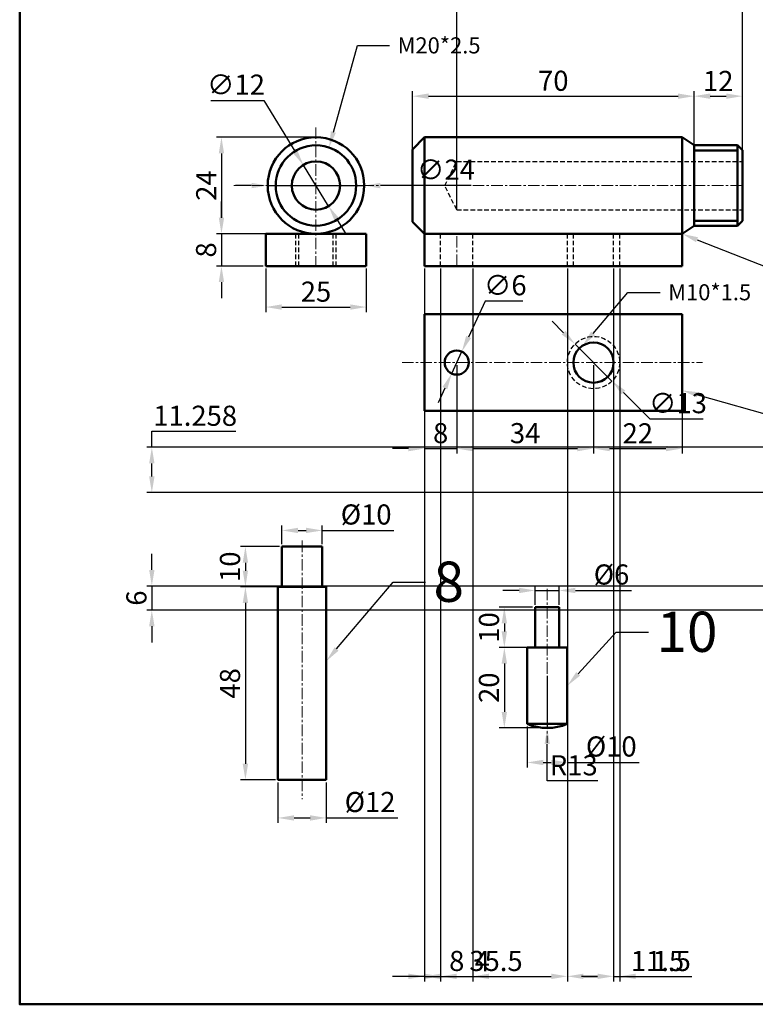
# Model space of a CAD drawing. Units: millimetres. Extents: x 24 to 508, y -182 to 223.
# Tile 1 of 6: x 24 to 207, y -182 to 63. Entities that reach past the tile are written whole.
import ezdxf
from ezdxf import colors
from ezdxf.entities.mleader import LeaderData, LeaderLine
from ezdxf.math import Vec2, Vec3

# ---------------------------------------------------------------- set-up
doc = ezdxf.new("R2010")
doc.units = ezdxf.units.MM
doc.header["$LTSCALE"] = 0.3
doc.linetypes.add('CENTER', pattern=[50.8, 31.75, -6.35, 6.35, -6.35])
doc.linetypes.add('DASHED', pattern=[19.05, 12.7, -6.35])
for name, color, linetype, lineweight in [('M-CNTR', 1, 'CENTER', 18), ('M-DIMS', 2, 'Continuous', 25), ('M-HIDN', 4, 'DASHED', 25), ('M-OUTL', 7, 'Continuous', 50)]:
    doc.layers.add(name, color=color, linetype=linetype, lineweight=lineweight)
doc.styles.get("Standard").update_dxf_attribs({"font": 'arial.ttf'})
doc.dimstyles.new('ISO-25', dxfattribs={"dimtxt": 5, "dimasz": 4, "dimexe": 1.25, "dimexo": 0.625, "dimtad": 1, "dimtoh": 1, "dimdec": 0, "dimtxsty": 'Standard', "dimcen": 2.5, "dimadec": 0, "dimazin": 0, "dimtfac": 1, "dimtdec": 0, "dimtmove": 0, "dimatfit": 3, "dimfxl": 1, "dimarcsym": 0})

# ---------------------------------------------------------------- blocks, each defined once
blk = doc.blocks.new('*D16')
at = {"layer": 'Defpoints', "color": 0, "ltscale": 0.3, "transparency": 16777216}
for p in [(191.36, 44.16), (121.36, 21.94), (191.36, 21.94)]:
    blk.add_point(p, dxfattribs=at)
at = {"layer": 'M-DIMS', "color": 0, "lineweight": -2, "ltscale": 0.3, "transparency": 16777216}
for p, q in [((121.36, 22.57), (121.36, 45.41)), ((125.36, 44.16), (187.36, 44.16)), ((191.36, 22.57), (191.36, 45.41))]:
    blk.add_line(p, q, dxfattribs=at)
at = {"layer": 'M-DIMS', "color": 0, "ltscale": 0.3, "transparency": 16777216}
for points in [[(125.36, 44.83), (125.36, 43.49), (121.36, 44.16)], [(187.36, 44.83), (187.36, 43.49), (191.36, 44.16)]]:
    blk.add_solid(points, dxfattribs=at)
at = {"layer": 'M-DIMS', "color": 0, "ltscale": 0.3, "transparency": 16777216, "insert": (156.36, 47.34), "char_height": 5, "attachment_point": 5}
blk.add_mtext('70', dxfattribs=at)
blk = doc.blocks.new('*D17')
at = {"layer": 'Defpoints', "color": 0, "ltscale": 0.3, "transparency": 16777216}
for p in [(203.36, 44.16), (191.36, 21.94), (203.36, 21.94)]:
    blk.add_point(p, dxfattribs=at)
at = {"layer": 'M-DIMS', "color": 0, "lineweight": -2, "ltscale": 0.3, "transparency": 16777216}
for p, q in [((191.36, 22.57), (191.36, 45.41)), ((195.36, 44.16), (199.36, 44.16)), ((203.36, 22.57), (203.36, 45.41))]:
    blk.add_line(p, q, dxfattribs=at)
at = {"layer": 'M-DIMS', "color": 0, "ltscale": 0.3, "transparency": 16777216}
for points in [[(195.36, 44.83), (195.36, 43.49), (191.36, 44.16)], [(199.36, 44.83), (199.36, 43.49), (203.36, 44.16)]]:
    blk.add_solid(points, dxfattribs=at)
at = {"layer": 'M-DIMS', "color": 0, "ltscale": 0.3, "transparency": 16777216, "insert": (197.36, 47.29), "char_height": 5, "attachment_point": 5}
blk.add_mtext('12', dxfattribs=at)
blk = doc.blocks.new('*D18')
at = {"layer": 'Defpoints', "color": 0, "ltscale": 0.3, "transparency": 16777216}
for p in [(84.87, 9.94), (73.88, 1.94), (84.87, 1.94)]:
    blk.add_point(p, dxfattribs=at)
at = {"layer": 'M-DIMS', "color": 0, "lineweight": -2, "ltscale": 0.3, "transparency": 16777216}
for p, q in [((73.88, 13.94), (73.88, 17.94)), ((84.24, 9.94), (72.63, 9.94)), ((73.88, 9.94), (73.88, 1.94)), ((84.24, 1.94), (72.63, 1.94)), ((73.88, -2.06), (73.88, -6.06))]:
    blk.add_line(p, q, dxfattribs=at)
at = {"layer": 'M-DIMS', "color": 0, "ltscale": 0.3, "transparency": 16777216}
for points in [[(73.21, 13.94), (74.54, 13.94), (73.88, 9.94)], [(73.21, -2.06), (74.54, -2.06), (73.88, 1.94)]]:
    blk.add_solid(points, dxfattribs=at)
at = {"layer": 'M-DIMS', "color": 0, "ltscale": 0.3, "transparency": 16777216, "insert": (70.7, 5.94), "char_height": 5, "attachment_point": 5, "rotation": 90}
blk.add_mtext('8', dxfattribs=at)
blk = doc.blocks.new('*D19')
at = {"layer": 'Defpoints', "color": 0, "ltscale": 0.3, "transparency": 16777216}
for p in [(97.37, 33.94), (73.88, 9.94), (97.37, 9.94)]:
    blk.add_point(p, dxfattribs=at)
at = {"layer": 'M-DIMS', "color": 0, "lineweight": -2, "ltscale": 0.3, "transparency": 16777216}
for p, q in [((96.74, 33.94), (72.63, 33.94)), ((73.88, 29.94), (73.88, 13.94)), ((96.74, 9.94), (72.63, 9.94))]:
    blk.add_line(p, q, dxfattribs=at)
at = {"layer": 'M-DIMS', "color": 0, "ltscale": 0.3, "transparency": 16777216}
for points in [[(73.21, 29.94), (74.54, 29.94), (73.88, 33.94)], [(73.21, 13.94), (74.54, 13.94), (73.88, 9.94)]]:
    blk.add_solid(points, dxfattribs=at)
at = {"layer": 'M-DIMS', "color": 0, "ltscale": 0.3, "transparency": 16777216, "insert": (70.74, 21.94), "char_height": 5, "attachment_point": 5, "rotation": 90}
blk.add_mtext('24', dxfattribs=at)
blk = doc.blocks.new('*D20')
at = {"layer": 'Defpoints', "color": 0, "ltscale": 0.3, "transparency": 16777216}
for p in [(84.87, 1.94), (109.87, 1.94), (109.87, -8.26)]:
    blk.add_point(p, dxfattribs=at)
at = {"layer": 'M-DIMS', "color": 0, "lineweight": -2, "ltscale": 0.3, "transparency": 16777216}
for p, q in [((84.87, 1.32), (84.87, -9.51)), ((109.87, 1.32), (109.87, -9.51)), ((88.87, -8.26), (105.87, -8.26))]:
    blk.add_line(p, q, dxfattribs=at)
at = {"layer": 'M-DIMS', "color": 0, "ltscale": 0.3, "transparency": 16777216}
for points in [[(88.87, -7.59), (88.87, -8.93), (84.87, -8.26)], [(105.87, -7.59), (105.87, -8.93), (109.87, -8.26)]]:
    blk.add_solid(points, dxfattribs=at)
at = {"layer": 'M-DIMS', "color": 0, "ltscale": 0.3, "transparency": 16777216, "insert": (97.37, -5.08), "char_height": 5, "attachment_point": 5}
blk.add_mtext('25', dxfattribs=at)
blk = doc.blocks.new('*D21')
at = {"layer": 'Defpoints', "color": 0, "ltscale": 0.3, "transparency": 16777216}
for p in [(94.23, 27.05), (100.51, 16.83)]:
    blk.add_point(p, dxfattribs=at)
at = {"layer": 'M-DIMS', "color": 0, "lineweight": -2, "ltscale": 0.3, "transparency": 16777216}
for p, q in [((71.21, 43.06), (84.39, 43.06)), ((84.39, 43.06), (92.13, 30.46)), ((100.51, 16.83), (94.23, 27.05)), ((102.6, 13.42), (104.7, 10.02))]:
    blk.add_line(p, q, dxfattribs=at)
at = {"layer": 'M-DIMS', "color": 0, "ltscale": 0.3, "transparency": 16777216}
for points in [[(92.7, 30.81), (91.56, 30.11), (94.23, 27.05)], [(103.17, 13.77), (102.04, 13.07), (100.51, 16.83)]]:
    blk.add_solid(points, dxfattribs=at)
at = {"layer": 'M-DIMS', "color": 0, "ltscale": 0.3, "transparency": 16777216, "insert": (77.49, 46.38), "char_height": 5, "attachment_point": 5}
blk.add_mtext('∅12', dxfattribs=at)
blk = doc.blocks.new('*D22')
at = {"layer": 'Defpoints', "color": 0, "ltscale": 0.3, "transparency": 16777216}
for p in [(132.36, -22.06), (124.36, -34.06), (132.36, -43.43)]:
    blk.add_point(p, dxfattribs=at)
at = {"layer": 'M-DIMS', "color": 0, "lineweight": -2, "ltscale": 0.3, "transparency": 16777216}
for p, q in [((132.36, -22.68), (132.36, -44.68)), ((124.36, -34.68), (124.36, -44.68)), ((120.36, -43.43), (116.36, -43.43)), ((124.36, -43.43), (132.36, -43.43)), ((136.36, -43.43), (140.36, -43.43))]:
    blk.add_line(p, q, dxfattribs=at)
at = {"layer": 'M-DIMS', "color": 0, "ltscale": 0.3, "transparency": 16777216}
for points in [[(120.36, -42.76), (120.36, -44.1), (124.36, -43.43)], [(136.36, -42.76), (136.36, -44.1), (132.36, -43.43)]]:
    blk.add_solid(points, dxfattribs=at)
at = {"layer": 'M-DIMS', "color": 0, "ltscale": 0.3, "transparency": 16777216, "insert": (128.36, -40.25), "char_height": 5, "attachment_point": 5}
blk.add_mtext('8', dxfattribs=at)
blk = doc.blocks.new('*D23')
at = {"layer": 'Defpoints', "color": 0, "ltscale": 0.3, "transparency": 16777216}
for p in [(166.36, -22.06), (132.36, -34.06), (166.36, -43.43)]:
    blk.add_point(p, dxfattribs=at)
at = {"layer": 'M-DIMS', "color": 0, "lineweight": -2, "ltscale": 0.3, "transparency": 16777216}
for p, q in [((166.36, -22.68), (166.36, -44.68)), ((132.36, -34.68), (132.36, -44.68)), ((136.36, -43.43), (162.36, -43.43))]:
    blk.add_line(p, q, dxfattribs=at)
at = {"layer": 'M-DIMS', "color": 0, "ltscale": 0.3, "transparency": 16777216}
for points in [[(136.36, -42.76), (136.36, -44.1), (132.36, -43.43)], [(162.36, -42.76), (162.36, -44.1), (166.36, -43.43)]]:
    blk.add_solid(points, dxfattribs=at)
at = {"layer": 'M-DIMS', "color": 0, "ltscale": 0.3, "transparency": 16777216, "insert": (149.36, -40.25), "char_height": 5, "attachment_point": 5}
blk.add_mtext('34', dxfattribs=at)
blk = doc.blocks.new('*D24')
at = {"layer": 'Defpoints', "color": 0, "ltscale": 0.3, "transparency": 16777216}
for p in [(166.36, -22.06), (188.36, -22.06), (188.36, -43.43)]:
    blk.add_point(p, dxfattribs=at)
at = {"layer": 'M-DIMS', "color": 0, "lineweight": -2, "ltscale": 0.3, "transparency": 16777216}
for p, q in [((166.36, -22.68), (166.36, -44.68)), ((188.36, -22.68), (188.36, -44.68)), ((170.36, -43.43), (184.36, -43.43))]:
    blk.add_line(p, q, dxfattribs=at)
at = {"layer": 'M-DIMS', "color": 0, "ltscale": 0.3, "transparency": 16777216}
for points in [[(170.36, -42.76), (170.36, -44.1), (166.36, -43.43)], [(184.36, -42.76), (184.36, -44.1), (188.36, -43.43)]]:
    blk.add_solid(points, dxfattribs=at)
at = {"layer": 'M-DIMS', "color": 0, "ltscale": 0.3, "transparency": 16777216, "insert": (177.36, -40.3), "char_height": 5, "attachment_point": 5}
blk.add_mtext('22', dxfattribs=at)
blk = doc.blocks.new('*D25')
at = {"layer": 'Defpoints', "color": 0, "ltscale": 0.3, "transparency": 16777216}
for p in [(133.62, -19.34), (131.1, -24.78)]:
    blk.add_point(p, dxfattribs=at)
at = {"layer": 'M-DIMS', "color": 0, "lineweight": -2, "ltscale": 0.3, "transparency": 16777216}
for p, q in [((139.44, -6.79), (135.3, -15.71)), ((148.78, -6.79), (139.44, -6.79)), ((131.1, -24.78), (133.62, -19.34)), ((129.41, -28.41), (127.73, -32.04))]:
    blk.add_line(p, q, dxfattribs=at)
at = {"layer": 'M-DIMS', "color": 0, "ltscale": 0.3, "transparency": 16777216}
for points in [[(134.7, -15.43), (135.91, -15.99), (133.62, -19.34)], [(128.81, -28.13), (130.02, -28.69), (131.1, -24.78)]]:
    blk.add_solid(points, dxfattribs=at)
at = {"layer": 'M-DIMS', "color": 0, "ltscale": 0.3, "transparency": 16777216, "insert": (144.42, -3.48), "char_height": 5, "attachment_point": 5}
blk.add_mtext('∅6', dxfattribs=at)
blk = doc.blocks.new('*D45')
at = {"layer": 'Defpoints', "color": 0, "ltscale": 0.3, "transparency": 16777216}
for p in [(88.92, -67.8), (79.83, -77.8), (88.92, -77.8)]:
    blk.add_point(p, dxfattribs=at)
at = {"layer": 'M-DIMS', "color": 0, "lineweight": -2, "ltscale": 0.3, "transparency": 16777216}
for p, q in [((88.29, -67.8), (78.58, -67.8)), ((79.83, -71.8), (79.83, -73.8)), ((88.29, -77.8), (78.58, -77.8))]:
    blk.add_line(p, q, dxfattribs=at)
at = {"layer": 'M-DIMS', "color": 0, "ltscale": 0.3, "transparency": 16777216}
for points in [[(79.16, -71.8), (80.49, -71.8), (79.83, -67.8)], [(79.16, -73.8), (80.49, -73.8), (79.83, -77.8)]]:
    blk.add_solid(points, dxfattribs=at)
at = {"layer": 'M-DIMS', "color": 0, "ltscale": 0.3, "transparency": 16777216, "insert": (76.65, -72.8), "char_height": 5, "attachment_point": 5, "rotation": 90}
blk.add_mtext('10', dxfattribs=at)
blk = doc.blocks.new('*D46')
at = {"layer": 'Defpoints', "color": 0, "ltscale": 0.3, "transparency": 16777216}
for p in [(87.92, -77.8), (79.83, -125.8), (87.92, -125.8)]:
    blk.add_point(p, dxfattribs=at)
at = {"layer": 'M-DIMS', "color": 0, "lineweight": -2, "ltscale": 0.3, "transparency": 16777216}
for p, q in [((87.29, -77.8), (78.58, -77.8)), ((79.83, -81.8), (79.83, -121.8)), ((87.29, -125.8), (78.58, -125.8))]:
    blk.add_line(p, q, dxfattribs=at)
at = {"layer": 'M-DIMS', "color": 0, "ltscale": 0.3, "transparency": 16777216}
for points in [[(79.16, -81.8), (80.49, -81.8), (79.83, -77.8)], [(79.16, -121.8), (80.49, -121.8), (79.83, -125.8)]]:
    blk.add_solid(points, dxfattribs=at)
at = {"layer": 'M-DIMS', "color": 0, "ltscale": 0.3, "transparency": 16777216, "insert": (76.65, -101.8), "char_height": 5, "attachment_point": 5, "rotation": 90}
blk.add_mtext('48', dxfattribs=at)
blk = doc.blocks.new('*D47')
at = {"layer": 'Defpoints', "color": 0, "ltscale": 0.3, "transparency": 16777216}
for p in [(87.92, -125.8), (99.92, -125.8), (99.92, -135.25)]:
    blk.add_point(p, dxfattribs=at)
at = {"layer": 'M-DIMS', "color": 0, "lineweight": -2, "ltscale": 0.3, "transparency": 16777216}
for p, q in [((87.92, -126.42), (87.92, -136.5)), ((99.92, -126.42), (99.92, -136.5)), ((91.92, -135.25), (95.92, -135.25)), ((99.92, -135.25), (117.72, -135.25))]:
    blk.add_line(p, q, dxfattribs=at)
at = {"layer": 'M-DIMS', "color": 0, "ltscale": 0.3, "transparency": 16777216}
for points in [[(91.92, -134.59), (91.92, -135.92), (87.92, -135.25)], [(95.92, -134.59), (95.92, -135.92), (99.92, -135.25)]]:
    blk.add_solid(points, dxfattribs=at)
at = {"layer": 'M-DIMS', "color": 0, "ltscale": 0.3, "transparency": 16777216, "insert": (110.82, -131.94), "char_height": 5, "attachment_point": 5}
blk.add_mtext('%%C12', dxfattribs=at)
blk = doc.blocks.new('*D48')
at = {"layer": 'Defpoints', "color": 0, "ltscale": 0.3, "transparency": 16777216}
for p in [(98.92, -63.79), (88.92, -67.8), (98.92, -67.8)]:
    blk.add_point(p, dxfattribs=at)
at = {"layer": 'M-DIMS', "color": 0, "lineweight": -2, "ltscale": 0.3, "transparency": 16777216}
for p, q in [((88.92, -67.17), (88.92, -62.54)), ((98.92, -67.17), (98.92, -62.54)), ((92.92, -63.79), (94.92, -63.79)), ((98.92, -63.79), (116.75, -63.79))]:
    blk.add_line(p, q, dxfattribs=at)
at = {"layer": 'M-DIMS', "color": 0, "ltscale": 0.3, "transparency": 16777216}
for points in [[(92.92, -63.12), (92.92, -64.45), (88.92, -63.79)], [(94.92, -63.12), (94.92, -64.45), (98.92, -63.79)]]:
    blk.add_solid(points, dxfattribs=at)
at = {"layer": 'M-DIMS', "color": 0, "ltscale": 0.3, "transparency": 16777216, "insert": (109.84, -60.47), "char_height": 5, "attachment_point": 5}
blk.add_mtext('%%C10', dxfattribs=at)
blk = doc.blocks.new('*D49')
at = {"layer": 'Defpoints', "color": 0, "ltscale": 0.3, "transparency": 16777216}
for p in [(157.85, -78.71), (151.85, -82.89), (157.85, -82.89)]:
    blk.add_point(p, dxfattribs=at)
at = {"layer": 'M-DIMS', "color": 0, "lineweight": -2, "ltscale": 0.3, "transparency": 16777216}
for p, q in [((151.85, -82.26), (151.85, -77.46)), ((157.85, -82.26), (157.85, -77.46)), ((147.85, -78.71), (143.85, -78.71)), ((151.85, -78.71), (157.85, -78.71)), ((161.85, -78.71), (175.81, -78.71))]:
    blk.add_line(p, q, dxfattribs=at)
at = {"layer": 'M-DIMS', "color": 0, "ltscale": 0.3, "transparency": 16777216}
for points in [[(147.85, -78.04), (147.85, -79.38), (151.85, -78.71)], [(161.85, -78.04), (161.85, -79.38), (157.85, -78.71)]]:
    blk.add_solid(points, dxfattribs=at)
at = {"layer": 'M-DIMS', "color": 0, "ltscale": 0.3, "transparency": 16777216, "insert": (170.83, -75.39), "char_height": 5, "attachment_point": 5}
blk.add_mtext('%%C6', dxfattribs=at)
blk = doc.blocks.new('*D50')
at = {"layer": 'Defpoints', "color": 0, "ltscale": 0.3, "transparency": 16777216}
for p in [(151.85, -82.89), (144.19, -92.89), (151.85, -92.89)]:
    blk.add_point(p, dxfattribs=at)
at = {"layer": 'M-DIMS', "color": 0, "lineweight": -2, "ltscale": 0.3, "transparency": 16777216}
for p, q in [((151.22, -82.89), (142.94, -82.89)), ((144.19, -86.89), (144.19, -88.89)), ((151.22, -92.89), (142.94, -92.89))]:
    blk.add_line(p, q, dxfattribs=at)
at = {"layer": 'M-DIMS', "color": 0, "ltscale": 0.3, "transparency": 16777216}
for points in [[(143.52, -86.89), (144.86, -86.89), (144.19, -82.89)], [(143.52, -88.89), (144.86, -88.89), (144.19, -92.89)]]:
    blk.add_solid(points, dxfattribs=at)
at = {"layer": 'M-DIMS', "color": 0, "ltscale": 0.3, "transparency": 16777216, "insert": (141.01, -87.89), "char_height": 5, "attachment_point": 5, "rotation": 90}
blk.add_mtext('10', dxfattribs=at)
blk = doc.blocks.new('*D51')
at = {"layer": 'Defpoints', "color": 0, "ltscale": 0.3, "transparency": 16777216}
for p in [(149.85, -92.89), (144.19, -112.89), (154.85, -112.89)]:
    blk.add_point(p, dxfattribs=at)
at = {"layer": 'M-DIMS', "color": 0, "lineweight": -2, "ltscale": 0.3, "transparency": 16777216}
for p, q in [((149.22, -92.89), (142.94, -92.89)), ((144.19, -96.89), (144.19, -108.89)), ((154.22, -112.89), (142.94, -112.89))]:
    blk.add_line(p, q, dxfattribs=at)
at = {"layer": 'M-DIMS', "color": 0, "ltscale": 0.3, "transparency": 16777216}
for points in [[(143.52, -96.89), (144.86, -96.89), (144.19, -92.89)], [(143.52, -108.89), (144.86, -108.89), (144.19, -112.89)]]:
    blk.add_solid(points, dxfattribs=at)
at = {"layer": 'M-DIMS', "color": 0, "ltscale": 0.3, "transparency": 16777216, "insert": (141.01, -102.89), "char_height": 5, "attachment_point": 5, "rotation": 90}
blk.add_mtext('20', dxfattribs=at)
blk = doc.blocks.new('*D52')
at = {"layer": 'Defpoints', "color": 0, "ltscale": 0.3, "transparency": 16777216}
for p in [(149.85, -111.89), (159.85, -111.89), (159.85, -121.46)]:
    blk.add_point(p, dxfattribs=at)
at = {"layer": 'M-DIMS', "color": 0, "lineweight": -2, "ltscale": 0.3, "transparency": 16777216}
for p, q in [((149.85, -112.51), (149.85, -122.71)), ((159.85, -112.51), (159.85, -122.71)), ((153.85, -121.46), (155.85, -121.46)), ((159.85, -121.46), (177.68, -121.46))]:
    blk.add_line(p, q, dxfattribs=at)
at = {"layer": 'M-DIMS', "color": 0, "ltscale": 0.3, "transparency": 16777216}
for points in [[(153.85, -120.8), (153.85, -122.13), (149.85, -121.46)], [(155.85, -120.8), (155.85, -122.13), (159.85, -121.46)]]:
    blk.add_solid(points, dxfattribs=at)
at = {"layer": 'M-DIMS', "color": 0, "ltscale": 0.3, "transparency": 16777216, "insert": (170.76, -118.14), "char_height": 5, "attachment_point": 5}
blk.add_mtext('%%C10', dxfattribs=at)
blk = doc.blocks.new('*D68')
at = {"layer": 'Defpoints', "color": 0, "ltscale": 0.3, "transparency": 16777216}
for p in [(203.36, 199.79), (132.36, 15.94), (203.36, 15.94)]:
    blk.add_point(p, dxfattribs=at)
at = {"layer": 'M-DIMS', "color": 0, "lineweight": -2, "ltscale": 0.3, "transparency": 16777216}
for p, q in [((132.36, 16.57), (132.36, 201.04)), ((203.36, 16.57), (203.36, 201.04)), ((136.36, 199.79), (199.36, 199.79))]:
    blk.add_line(p, q, dxfattribs=at)
at = {"layer": 'M-DIMS', "color": 0, "ltscale": 0.3, "transparency": 16777216}
for points in [[(136.36, 200.46), (136.36, 199.12), (132.36, 199.79)], [(199.36, 200.46), (199.36, 199.12), (203.36, 199.79)]]:
    blk.add_solid(points, dxfattribs=at)
at = {"layer": 'M-DIMS', "color": 0, "ltscale": 0.3, "transparency": 16777216, "insert": (167.86, 202.93), "char_height": 5, "attachment_point": 5}
blk.add_mtext('71', dxfattribs=at)
blk = doc.blocks.new('*D69')
at = {"layer": 'Defpoints', "color": 0, "ltscale": 0.3, "transparency": 16777216}
for p in [(124.36, 1.94), (128.36, 1.94), (128.36, -174.63)]:
    blk.add_point(p, dxfattribs=at)
at = {"layer": 'M-DIMS', "color": 0, "lineweight": -2, "ltscale": 0.3, "transparency": 16777216}
for p, q in [((124.36, 1.32), (124.36, -175.88)), ((128.36, 1.32), (128.36, -175.88)), ((120.36, -174.63), (116.36, -174.63)), ((124.36, -174.63), (128.36, -174.63)), ((132.36, -174.63), (141.07, -174.63))]:
    blk.add_line(p, q, dxfattribs=at)
at = {"layer": 'M-DIMS', "color": 0, "ltscale": 0.3, "transparency": 16777216}
for points in [[(120.36, -173.96), (120.36, -175.3), (124.36, -174.63)], [(132.36, -173.96), (132.36, -175.3), (128.36, -174.63)]]:
    blk.add_solid(points, dxfattribs=at)
at = {"layer": 'M-DIMS', "color": 0, "ltscale": 0.3, "transparency": 16777216, "insert": (138.71, -171.51), "char_height": 5, "attachment_point": 5}
blk.add_mtext('4', dxfattribs=at)
blk = doc.blocks.new('*D70')
at = {"layer": 'Defpoints', "color": 0, "ltscale": 0.3, "transparency": 16777216}
for p in [(128.36, 1.94), (136.36, 1.94), (136.36, -174.63)]:
    blk.add_point(p, dxfattribs=at)
at = {"layer": 'M-DIMS', "color": 0, "lineweight": -2, "ltscale": 0.3, "transparency": 16777216}
for p, q in [((128.36, 1.32), (128.36, -175.88)), ((136.36, 1.32), (136.36, -175.88)), ((124.36, -174.63), (120.36, -174.63)), ((128.36, -174.63), (136.36, -174.63)), ((140.36, -174.63), (144.36, -174.63))]:
    blk.add_line(p, q, dxfattribs=at)
at = {"layer": 'M-DIMS', "color": 0, "ltscale": 0.3, "transparency": 16777216}
for points in [[(124.36, -173.96), (124.36, -175.3), (128.36, -174.63)], [(140.36, -173.96), (140.36, -175.3), (136.36, -174.63)]]:
    blk.add_solid(points, dxfattribs=at)
at = {"layer": 'M-DIMS', "color": 0, "ltscale": 0.3, "transparency": 16777216, "insert": (132.36, -171.45), "char_height": 5, "attachment_point": 5}
blk.add_mtext('8', dxfattribs=at)
blk = doc.blocks.new('*D71')
at = {"layer": 'Defpoints', "color": 0, "ltscale": 0.3, "transparency": 16777216}
for p in [(124.36, 1.94), (159.86, 1.94), (159.86, -174.63)]:
    blk.add_point(p, dxfattribs=at)
at = {"layer": 'M-DIMS', "color": 0, "lineweight": -2, "ltscale": 0.3, "transparency": 16777216}
for p, q in [((124.36, 1.32), (124.36, -175.88)), ((159.86, 1.32), (159.86, -175.88)), ((128.36, -174.63), (155.86, -174.63))]:
    blk.add_line(p, q, dxfattribs=at)
at = {"layer": 'M-DIMS', "color": 0, "ltscale": 0.3, "transparency": 16777216}
for points in [[(128.36, -173.96), (128.36, -175.3), (124.36, -174.63)], [(155.86, -173.96), (155.86, -175.3), (159.86, -174.63)]]:
    blk.add_solid(points, dxfattribs=at)
at = {"layer": 'M-DIMS', "color": 0, "ltscale": 0.3, "transparency": 16777216, "insert": (142.11, -171.45), "char_height": 5, "attachment_point": 5}
blk.add_mtext('35.5', dxfattribs=at)
blk = doc.blocks.new('*D72')
at = {"layer": 'Defpoints', "color": 0, "ltscale": 0.3, "transparency": 16777216}
for p in [(159.86, 1.94), (171.36, 1.94), (171.36, -174.63)]:
    blk.add_point(p, dxfattribs=at)
at = {"layer": 'M-DIMS', "color": 0, "lineweight": -2, "ltscale": 0.3, "transparency": 16777216}
for p, q in [((159.86, 1.32), (159.86, -175.88)), ((171.36, 1.32), (171.36, -175.88)), ((163.86, -174.63), (167.36, -174.63)), ((171.36, -174.63), (189.16, -174.63))]:
    blk.add_line(p, q, dxfattribs=at)
at = {"layer": 'M-DIMS', "color": 0, "ltscale": 0.3, "transparency": 16777216}
for points in [[(163.86, -173.96), (163.86, -175.3), (159.86, -174.63)], [(167.36, -173.96), (167.36, -175.3), (171.36, -174.63)]]:
    blk.add_solid(points, dxfattribs=at)
at = {"layer": 'M-DIMS', "color": 0, "ltscale": 0.3, "transparency": 16777216, "insert": (182.26, -171.45), "char_height": 5, "attachment_point": 5}
blk.add_mtext('11.5', dxfattribs=at)
blk = doc.blocks.new('*D73')
at = {"layer": 'Defpoints', "color": 0, "ltscale": 0.3, "transparency": 16777216}
for p in [(171.36, 1.94), (172.86, 1.94), (172.86, -174.63)]:
    blk.add_point(p, dxfattribs=at)
at = {"layer": 'M-DIMS', "color": 0, "lineweight": -2, "ltscale": 0.3, "transparency": 16777216}
for p, q in [((171.36, 1.32), (171.36, -175.88)), ((172.86, 1.32), (172.86, -175.88)), ((167.36, -174.63), (163.36, -174.63)), ((171.36, -174.63), (172.86, -174.63)), ((176.86, -174.63), (190.78, -174.63))]:
    blk.add_line(p, q, dxfattribs=at)
at = {"layer": 'M-DIMS', "color": 0, "ltscale": 0.3, "transparency": 16777216}
for points in [[(167.36, -173.96), (167.36, -175.3), (171.36, -174.63)], [(176.86, -173.96), (176.86, -175.3), (172.86, -174.63)]]:
    blk.add_solid(points, dxfattribs=at)
at = {"layer": 'M-DIMS', "color": 0, "ltscale": 0.3, "transparency": 16777216, "insert": (185.82, -171.45), "char_height": 5, "attachment_point": 5}
blk.add_mtext('1.5', dxfattribs=at)
blk = doc.blocks.new('*D76')
at = {"layer": 'Defpoints', "color": 0, "ltscale": 0.3, "transparency": 16777216}
for p in [(411.13, -77.61), (56.57, -83.61), (411.13, -83.61)]:
    blk.add_point(p, dxfattribs=at)
at = {"layer": 'M-DIMS', "color": 0, "lineweight": -2, "ltscale": 0.3, "transparency": 16777216}
for p, q in [((56.57, -73.61), (56.57, -69.61)), ((410.51, -77.61), (55.32, -77.61)), ((56.57, -77.61), (56.57, -83.61)), ((410.51, -83.61), (55.32, -83.61)), ((56.57, -87.61), (56.57, -91.61))]:
    blk.add_line(p, q, dxfattribs=at)
at = {"layer": 'M-DIMS', "color": 0, "ltscale": 0.3, "transparency": 16777216}
for points in [[(55.9, -73.61), (57.24, -73.61), (56.57, -77.61)], [(55.9, -87.61), (57.24, -87.61), (56.57, -83.61)]]:
    blk.add_solid(points, dxfattribs=at)
at = {"layer": 'M-DIMS', "color": 0, "ltscale": 0.3, "transparency": 16777216, "insert": (53.39, -80.61), "char_height": 5, "attachment_point": 5, "rotation": 90}
blk.add_mtext('6', dxfattribs=at)
blk = doc.blocks.new('*D77')
at = {"layer": 'Defpoints', "color": 0, "ltscale": 0.3, "transparency": 16777216}
for p in [(56.57, -43.11), (338.8, -43.11), (345.3, -54.37)]:
    blk.add_point(p, dxfattribs=at)
at = {"layer": 'M-DIMS', "color": 0, "lineweight": -2, "ltscale": 0.3, "transparency": 16777216}
for p, q in [((56.57, -43.11), (56.57, -39.11)), ((56.57, -39.11), (77.49, -39.11)), ((338.18, -43.11), (55.32, -43.11)), ((56.57, -50.37), (56.57, -47.11)), ((344.68, -54.37), (55.32, -54.37))]:
    blk.add_line(p, q, dxfattribs=at)
at = {"layer": 'M-DIMS', "color": 0, "ltscale": 0.3, "transparency": 16777216}
for points in [[(55.9, -47.11), (57.24, -47.11), (56.57, -43.11)], [(55.9, -50.37), (57.24, -50.37), (56.57, -54.37)]]:
    blk.add_solid(points, dxfattribs=at)
at = {"layer": 'M-DIMS', "color": 0, "ltscale": 0.3, "transparency": 16777216, "insert": (67.34, -35.93), "char_height": 5, "attachment_point": 5}
blk.add_mtext('11.258', dxfattribs=at)
blk = doc.blocks.new('*D81')
at = {"layer": 'Defpoints', "color": 0, "ltscale": 0.3, "transparency": 16777216}
for p in [(85.37, 21.95), (109.37, 21.94)]:
    blk.add_point(p, dxfattribs=at)
at = {"layer": 'M-DIMS', "color": 0, "lineweight": -2, "ltscale": 0.3, "transparency": 16777216}
for p, q in [((81.37, 21.95), (77.37, 21.95)), ((85.37, 21.95), (109.37, 21.94)), ((122.75, 21.94), (113.37, 21.94)), ((135.96, 21.94), (122.75, 21.94))]:
    blk.add_line(p, q, dxfattribs=at)
at = {"layer": 'M-DIMS', "color": 0, "ltscale": 0.3, "transparency": 16777216}
for points in [[(81.37, 22.61), (81.37, 21.28), (85.37, 21.95)], [(113.37, 22.61), (113.37, 21.27), (109.37, 21.94)]]:
    blk.add_solid(points, dxfattribs=at)
at = {"layer": 'M-DIMS', "color": 0, "ltscale": 0.3, "transparency": 16777216, "insert": (129.67, 25.25), "char_height": 5, "attachment_point": 5}
blk.add_mtext('∅24', dxfattribs=at)
blk = doc.blocks.new('*D82')
at = {"layer": 'Defpoints', "color": 0, "ltscale": 0.3, "transparency": 16777216}
for p in [(161.76, -17.46), (170.95, -26.65)]:
    blk.add_point(p, dxfattribs=at)
at = {"layer": 'M-DIMS', "color": 0, "lineweight": -2, "ltscale": 0.3, "transparency": 16777216}
for p, q in [((158.93, -14.63), (156.11, -11.8)), ((161.76, -17.46), (170.95, -26.65)), ((180.42, -36.12), (173.78, -29.48)), ((193.65, -36.12), (180.42, -36.12))]:
    blk.add_line(p, q, dxfattribs=at)
at = {"layer": 'M-DIMS', "color": 0, "ltscale": 0.3, "transparency": 16777216}
for points in [[(159.41, -14.16), (158.46, -15.1), (161.76, -17.46)], [(174.25, -29.01), (173.31, -29.95), (170.95, -26.65)]]:
    blk.add_solid(points, dxfattribs=at)
at = {"layer": 'M-DIMS', "color": 0, "ltscale": 0.3, "transparency": 16777216, "insert": (187.34, -32.8), "char_height": 5, "attachment_point": 5}
blk.add_mtext('∅13', dxfattribs=at)
blk = doc.blocks.new('*D88')
at = {"layer": 'Defpoints', "color": 0, "ltscale": 0.3, "transparency": 16777216}
for p in [(154.85, -99.89), (154.85, -112.89)]:
    blk.add_point(p, dxfattribs=at)
at = {"layer": 'M-DIMS', "color": 0, "lineweight": -2, "ltscale": 0.3, "transparency": 16777216}
for p, q in [((154.85, -99.89), (154.85, -112.89)), ((154.85, -126), (154.85, -116.89)), ((167.42, -126), (154.85, -126))]:
    blk.add_line(p, q, dxfattribs=at)
at = {"layer": 'M-DIMS', "color": 0, "ltscale": 0.3, "transparency": 16777216}
blk.add_solid([(155.51, -116.89), (154.18, -116.89), (154.85, -112.89)], dxfattribs=at)
at = {"layer": 'M-DIMS', "color": 0, "ltscale": 0.3, "transparency": 16777216, "insert": (161.45, -122.82), "char_height": 5, "attachment_point": 5}
blk.add_mtext('R13', dxfattribs=at)

msp = doc.modelspace()

# ---------------------------------------------------------------- linework, layer by layer
at = {"layer": 'M-CNTR', "ltscale": 0.3}
for p, q in [((97.3684, 36.3892), (97.3684, 1.9426)), ((76.9204, 21.9426), (203.3582, 21.9426)), ((132.3582, 1.9426), (132.3582, 9.9426)), ((118.7683, -22.0574), (193.4338, -22.0574)), ((93.9175, -66.3216), (93.9175, -130.5798)), ((154.8466, -78.2625), (154.8466, -116.6052))]:
    msp.add_line(p, q, dxfattribs=at)
at = {"layer": 'M-HIDN', "ltscale": 0.3}
for p, q in [((129.3582, 21.9426), (132.3582, 27.9426)), ((132.3582, 27.9426), (203.3582, 27.9426)), ((132.3582, 15.9426), (132.3582, 27.9426)), ((132.3582, 15.9426), (129.3582, 21.9426)), ((132.3582, 15.9426), (203.3582, 15.9426)), ((92.3684, 1.9426), (92.3684, 9.9426)), ((93.1184, 1.9426), (93.1184, 9.9426)), ((101.6184, 1.9426), (101.6184, 9.9426)), ((102.3684, 1.9426), (102.3684, 9.9426)), ((128.3582, 1.9426), (128.3582, 9.9426)), ((136.3582, 1.9426), (136.3582, 9.9426)), ((159.8582, 1.9426), (159.8582, 9.9426)), ((161.3582, 1.9426), (161.3582, 9.9426)), ((171.3582, 1.9426), (171.3582, 9.9426)), ((172.8582, 1.9426), (172.8582, 9.9426))]:
    msp.add_line(p, q, dxfattribs=at)
msp.add_circle((166.3582, -22.0574), 6.5, dxfattribs=at)
at = {"layer": 'M-OUTL', "ltscale": 0.3}
for p, q in [((121.3582, 30.9426), (124.3582, 33.9426)), ((124.3582, 33.9426), (188.3582, 33.9426)), ((124.3582, 33.9426), (124.3582, 9.9426)), ((188.3582, 33.9426), (188.3582, 9.9426)), ((191.3582, 31.9426), (188.3582, 33.9426)), ((191.3582, 31.9426), (202.1582, 31.9426)), ((191.3582, 31.9426), (191.3582, 11.9426)), ((202.1582, 31.9426), (203.3582, 30.7426)), ((202.1582, 31.9426), (202.1582, 11.9426)), ((121.3582, 30.9426), (121.3582, 12.9426)), ((191.3582, 30.6926), (202.1582, 30.6926)), ((203.3582, 30.7426), (203.3582, 13.1426)), ((121.3582, 12.9426), (124.3582, 9.9426)), ((191.3582, 13.1926), (202.1582, 13.1926)), ((203.3582, 13.1426), (202.1582, 11.9426)), ((109.8684, 9.9426), (84.8684, 9.9426)), ((84.8684, 9.9426), (84.8684, 1.9426)), ((109.8684, 9.9426), (109.8684, 1.9426)), ((188.3582, 9.9426), (124.3582, 9.9426)), ((124.3582, 9.9426), (124.3582, 1.9426)), ((188.3582, 9.9426), (191.3582, 11.9426)), ((188.3582, 1.9426), (188.3582, 9.9426)), ((191.3582, 11.9426), (202.1582, 11.9426)), ((109.8684, 1.9426), (84.8684, 1.9426)), ((124.3582, 1.9426), (188.3582, 1.9426)), ((124.3582, -10.0574), (188.3582, -10.0574)), ((124.3582, -10.0574), (124.3582, -34.0574)), ((188.3582, -34.0574), (188.3582, -10.0574)), ((124.3582, -34.0574), (188.3582, -34.0574)), ((88.9175, -67.7966), (98.9175, -67.7966)), ((88.9175, -77.7966), (88.9175, -67.7966)), ((98.9175, -67.7966), (98.9175, -77.7966)), ((87.9175, -125.7966), (87.9175, -77.7966)), ((87.9175, -77.7966), (88.9175, -77.7966)), ((88.9175, -77.7966), (99.9175, -77.7966)), ((99.9175, -77.7966), (99.9175, -125.7966)), ((151.8466, -82.8875), (157.8466, -82.8875)), ((151.8466, -92.8875), (151.8466, -82.8875)), ((157.8466, -82.8875), (157.8466, -92.8875)), ((149.8466, -111.8875), (149.8466, -92.8875)), ((149.8466, -92.8875), (151.8466, -92.8875)), ((151.8466, -92.8875), (159.8466, -92.8875)), ((159.8466, -92.8875), (159.8466, -111.8875)), ((159.8466, -111.8875), (149.8466, -111.8875)), ((99.9175, -125.7966), (87.9175, -125.7966))]:
    msp.add_line(p, q, dxfattribs=at)
msp.add_lwpolyline([(23.7253, 222.7463), (508.4225, 222.7463), (508.4225, -181.5799), (23.7253, -181.5799)], close=True, dxfattribs=at)
for centre, radius in [((97.3684, 21.9426), 12), ((97.3684, 21.9426), 10), ((97.3684, 21.9426), 6), ((166.3582, -22.0574), 5), ((132.3582, -22.0574), 3)]:
    msp.add_circle(centre, radius, dxfattribs=at)
msp.add_arc((154.8466, -99.8875), 13, 247.380135, 292.619865, dxfattribs=at)

# ---------------------------------------------------------------- dimensions: what is measured, and where the dimension line sits
at = {"layer": 'M-DIMS', "ltscale": 0.3}
for base, p1, p2, override, picture, middle in [((203.3582, 199.7903), (132.3582, 15.9426), (203.3582, 15.9426), {"dimdec": 0, "dimlfac": 1, "dimrnd": 0, "dimzin": 0, "dimdsep": 46, "dimlunit": 2}, '*D68', (167.8582, 202.9256)), ((191.3582, 44.1587), (121.3582, 21.9426), (191.3582, 21.9426), {"dimclrd": 0, "dimclre": 0, "dimclrt": 0}, '*D16', (156.3582, 47.3366)), ((203.3582, 44.1587), (191.3582, 21.9426), (203.3582, 21.9426), {"dimclrd": 0, "dimclre": 0, "dimclrt": 0}, '*D17', (197.3582, 47.294)), ((109.8684, -8.2593), (84.8684, 1.9426), (109.8684, 1.9426), {"dimclrd": 0, "dimclre": 0, "dimclrt": 0}, '*D20', (97.3684, -5.0814)), ((128.3582, -174.6307), (124.3582, 1.9426), (128.3582, 1.9426), {"dimdec": 0, "dimlfac": 1, "dimrnd": 0, "dimzin": 0, "dimdsep": 46, "dimlunit": 2}, '*D69', (138.7124, -171.5057)), ((136.3582, -174.6307), (128.3582, 1.9426), (136.3582, 1.9426), {"dimdec": 0, "dimlfac": 1, "dimrnd": 0, "dimzin": 0, "dimdsep": 46, "dimlunit": 2}, '*D70', (132.3582, -171.4528)), ((159.8582, -174.6307), (124.3582, 1.9426), (159.8582, 1.9426), {"dimdec": 1, "dimlfac": 1, "dimrnd": 0, "dimzin": 0, "dimdsep": 46, "dimlunit": 2}, '*D71', (142.1082, -171.4511)), ((171.3582, -174.6307), (159.8582, 1.9426), (171.3582, 1.9426), {"dimdec": 1, "dimlfac": 1, "dimrnd": 0, "dimzin": 0, "dimdsep": 46, "dimlunit": 2}, '*D72', (182.2605, -171.4528)), ((172.8582, -174.6307), (171.3582, 1.9426), (172.8582, 1.9426), {"dimdec": 1, "dimlfac": 1, "dimrnd": 0, "dimzin": 0, "dimdsep": 46, "dimlunit": 2}, '*D73', (185.8182, -171.4528)), ((132.3582, -43.4316), (124.3582, -34.0574), (132.3582, -22.0574), {"dimclrd": 0, "dimclre": 0, "dimclrt": 0}, '*D22', (128.3582, -40.2537)), ((166.3582, -43.4316), (132.3582, -34.0574), (166.3582, -22.0574), {"dimclrd": 0, "dimclre": 0, "dimclrt": 0}, '*D23', (149.3582, -40.252)), ((188.3582, -43.4316), (166.3582, -22.0574), (188.3582, -22.0574), {"dimclrd": 0, "dimclre": 0, "dimclrt": 0}, '*D24', (177.3582, -40.2964))]:
    dim = msp.add_linear_dim(base=base, p1=p1, p2=p2, dimstyle='ISO-25', override=override, dxfattribs=at)
    dim.commit()
    dim.dimension.update_dxf_attribs({"geometry": picture, "text_midpoint": middle})
for p1, p2, override, picture, middle in [((100.5102, 16.8309), (94.2266, 27.0543), {"dimclrd": 0, "dimclre": 0, "dimclrt": 0}, '*D21', (77.4863, 43.0633)), ((131.096, -24.779), (133.6205, -19.3359), {"dimclrd": 0, "dimclre": 0, "dimclrt": 0}, '*D25', (144.4199, -6.7928)), ((161.7625, -17.4608), (170.954, -26.654), {"dimdec": 0, "dimlfac": 1, "dimrnd": 0, "dimzin": 0, "dimdsep": 46, "dimlunit": 2}, '*D82', (187.3442, -36.1198))]:
    dim = msp.add_diameter_dim_2p(p1=p1, p2=p2, dimstyle='ISO-25', override=override, dxfattribs=at)
    dim.commit()
    dim.dimension.update_dxf_attribs({"geometry": picture, "text_midpoint": middle, "dimtype": 163})
for base, p1, p2, override, picture, middle in [((73.8754, 9.9426), (97.3684, 33.9426), (97.3684, 9.9426), {"dimclrd": 0, "dimclre": 0, "dimclrt": 0}, '*D19', (70.7401, 21.9426)), ((73.8754, 1.9426), (84.8684, 9.9426), (84.8684, 1.9426), {"dimclrd": 0, "dimclre": 0, "dimclrt": 0}, '*D18', (70.6975, 5.9426)), ((56.5704, -43.1068), (345.3004, -54.3651), (338.8004, -43.1068), {"dimdec": 3, "dimlfac": 1, "dimrnd": 0, "dimzin": 0, "dimdsep": 46, "dimlunit": 2}, '*D77', (67.3438, -35.9289)), ((79.8272, -77.7966), (88.9175, -67.7966), (88.9175, -77.7966), {"dimclrd": 0, "dimclre": 0, "dimclrt": 0}, '*D45', (76.6494, -72.7966)), ((56.5704, -83.6068), (411.1321, -77.6068), (411.1321, -83.6068), {"dimdec": 0, "dimlfac": 1, "dimrnd": 0, "dimzin": 0, "dimdsep": 46, "dimlunit": 2}, '*D76', (53.3925, -80.6068)), ((79.8272, -125.7966), (87.9175, -77.7966), (87.9175, -125.7966), {"dimclrd": 0, "dimclre": 0, "dimclrt": 0}, '*D46', (76.6494, -101.7966)), ((144.1884, -92.8875), (151.8466, -82.8875), (151.8466, -92.8875), {"dimclrd": 0, "dimclre": 0, "dimclrt": 0}, '*D50', (141.0106, -87.8875)), ((144.1884, -112.8875), (149.8466, -92.8875), (154.8466, -112.8875), {"dimclrd": 0, "dimclre": 0, "dimclrt": 0}, '*D51', (141.0106, -102.8875))]:
    dim = msp.add_linear_dim(base=base, p1=p1, p2=p2, angle=90, dimstyle='ISO-25', override=override, dxfattribs=at)
    dim.commit()
    dim.dimension.update_dxf_attribs({"geometry": picture, "text_midpoint": middle})
dim = msp.add_diameter_dim_2p(p1=(85.3684, 21.9452), p2=(109.3684, 21.94), dimstyle='ISO-25', override={"dimdec": 0, "dimlfac": 1, "dimrnd": 0, "dimzin": 0, "dimdsep": 46, "dimlunit": 2}, dxfattribs=at)
dim.commit()
dim.dimension.update_dxf_attribs({"geometry": '*D81', "text_midpoint": (122.7538, 21.9371)})
for base, p1, p2, picture, middle in [((98.9175, -63.7852), (88.9175, -67.7966), (98.9175, -67.7966), '*D48', (109.8351, -60.4675)), ((157.8466, -78.7092), (151.8466, -82.8875), (157.8466, -82.8875), '*D49', (170.8287, -75.3915)), ((159.8466, -121.4626), (149.8466, -111.8875), (159.8466, -111.8875), '*D52', (170.7643, -118.1449)), ((99.9175, -135.2544), (87.9175, -125.7966), (99.9175, -125.7966), '*D47', (110.818, -131.9367))]:
    dim = msp.add_linear_dim(base=base, p1=p1, p2=p2, text='%%C<>', dimstyle='ISO-25', override={"dimclrd": 0, "dimclre": 0, "dimclrt": 0}, dxfattribs=at)
    dim.commit()
    dim.dimension.update_dxf_attribs({"geometry": picture, "text_midpoint": middle})
dim = msp.add_radius_dim(center=(154.8466, -99.8875), mpoint=(154.847, -112.8875), dimstyle='ISO-25', override={"dimdec": 0, "dimlfac": 1, "dimrnd": 0, "dimzin": 0, "dimdsep": 46, "dimlunit": 2}, dxfattribs=at)
dim.commit()
dim.dimension.update_dxf_attribs({"geometry": '*D88', "text_midpoint": (161.4461, -122.8171)})

# ---------------------------------------------------------------- leaders
ml = msp.add_multileader_mtext('Standard', dxfattribs=at)
ml.set_content('M20*2.5', color=256)
ml.set_leader_properties()
ml.build(insert=Vec2(0, 0))
ctx = ml.context
ctx.base_point, ctx.plane_origin = Vec3(115.663, 56.75), Vec3(100.6317, 31.3951)
notes = []
notes.append((ctx, [(0, (1, 1, 0), (107.663, 56.75), (1, 0), 8, [(0, [(100.6317, 31.3951)], 0, [])])]))
ctx.mtext.insert, ctx.mtext.flow_direction = Vec3(117.663, 58.7841), 5
ml = msp.add_multileader_mtext('Standard', dxfattribs=at)
ml.set_content('5', color=256)
ml.set_leader_properties()
ml.build(insert=Vec2(0, 0))
ctx = ml.context
ctx.base_point, ctx.char_height, ctx.plane_origin = Vec3(226.7556, -2.0023), 10, Vec3(190.3582, 7.9426)
notes.append((ctx, [(0, (1, 1, 0), (218.7556, -2.0023), (1, 0), 8, [(0, [(188.3582, 9.9426)], 0, [])])]))
ctx.mtext.insert, ctx.mtext.flow_direction = Vec3(228.7556, 3.083), 5
ml = msp.add_multileader_mtext('Standard', dxfattribs=at)
ml.set_content('M10*1.5', color=256)
ml.set_leader_properties()
ml.build(insert=Vec2(0, 0))
ctx = ml.context
ctx.base_point, ctx.plane_origin = Vec3(182.9244, -4.6139), Vec3(163.6559, -17.8506)
notes.append((ctx, [(1, (1, 1, 0), (174.9244, -4.6139), (1, 0), 8, [(0, [(163.6559, -17.8506)], 0, [])])]))
ctx.mtext.insert, ctx.mtext.flow_direction = Vec3(184.9244, -2.5798), 5
ml = msp.add_multileader_mtext('Standard', dxfattribs=at)
ml.set_content('2', color=256)
ml.set_leader_properties()
ml.build(insert=Vec2(0, 0))
ctx = ml.context
ctx.base_point, ctx.char_height, ctx.plane_origin = Vec3(227.8339, -37.8459), 10, Vec3(188.3582, -28.9708)
notes.append((ctx, [(0, (1, 1, 0), (219.8339, -37.8459), (1, 0), 8, [(0, [(188.3582, -28.9708)], 0, [])])]))
ctx.mtext.insert, ctx.mtext.flow_direction = Vec3(229.8339, -32.8459), 5
ml = msp.add_multileader_mtext('Standard', dxfattribs=at)
ml.set_content('8', color=256)
ml.set_leader_properties()
ml.build(insert=Vec2(0, 0))
ctx = ml.context
ctx.base_point, ctx.char_height, ctx.plane_origin = Vec3(124.5843, -76.623), 10, Vec3(99.9175, -96.2929)
notes.append((ctx, [(0, (1, 1, 0), (116.5843, -76.623), (1, 0), 8, [(0, [(99.9175, -96.2929)], 0, [])])]))
ctx.mtext.insert, ctx.mtext.flow_direction = Vec3(126.5843, -71.5378), 5
ml = msp.add_multileader_mtext('Standard', dxfattribs=at)
ml.set_content('10', color=256)
ml.set_leader_properties()
ml.build(insert=Vec2(0, 0))
ctx = ml.context
ctx.base_point, ctx.char_height, ctx.plane_origin = Vec3(180.0198, -89.0624), 10, Vec3(159.8466, -102.3875)
notes.append((ctx, [(0, (1, 1, 0), (172.0198, -89.0624), (1, 0), 8, [(0, [(159.8466, -102.3875)], 0, [])])]))
ctx.mtext.insert, ctx.mtext.flow_direction = Vec3(182.0198, -83.9771), 5
for ctx, leaders in notes:
    for number, flags, end, landing, length, lines in leaders:
        leader = LeaderData()
        leader.index, (leader.has_last_leader_line, leader.has_dogleg_vector, leader.attachment_direction) = number, flags
        leader.last_leader_point, leader.dogleg_vector, leader.dogleg_length = Vec3(end), Vec3(landing), length
        for number, points, colour, breaks in lines:
            line = LeaderLine()
            line.index, line.vertices, line.color, line.breaks = number, Vec3.list(points), colors.encode_raw_color(colour), breaks
            leader.lines.append(line)
        ctx.leaders.append(leader)

doc.saveas('drawing.dxf')
